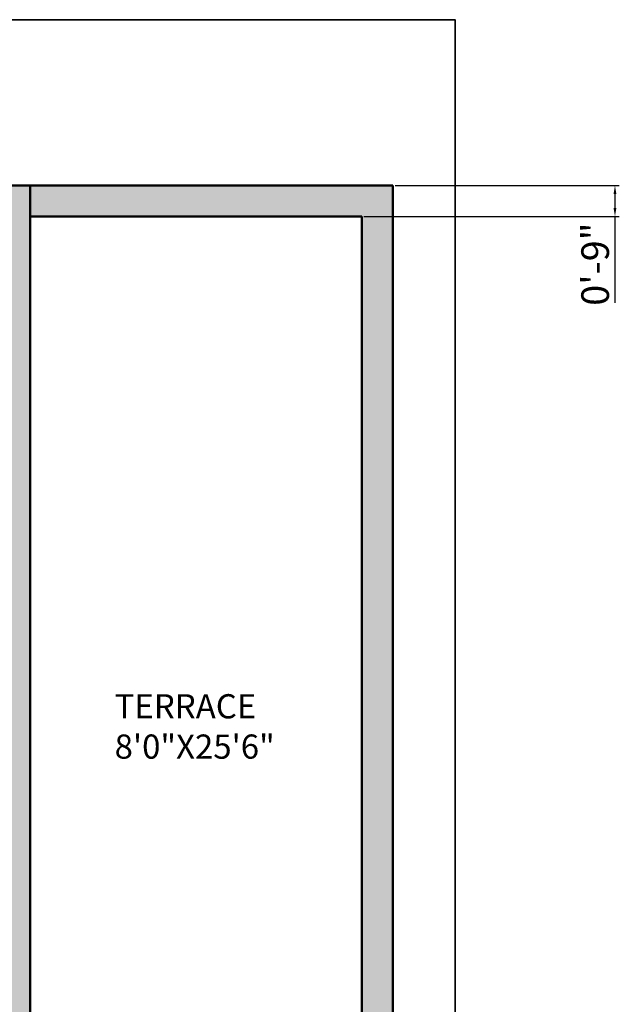
# Model space of a CAD drawing. Units: inches. Extents: x 1986 to 21484, y -1816 to 2016.
# Tile 45 of 85: x 2734 to 2908, y 1616 to 1901. Entities that reach past the tile are written whole.
import ezdxf

# ---------------------------------------------------------------- set-up
doc = ezdxf.new("R2010")
doc.units = ezdxf.units.IN
for name, color, linetype, lineweight in [('A-ANNO-DIMS', 2, 'Continuous', 18), ('A-AREA-IDEN', 3, 'Continuous', 18), ('A-WALL', 7, 'Continuous', 50), ('A-WALL-PATT', 8, 'Continuous', 13), ('C-PROP', 7, 'Continuous', 35)]:
    doc.layers.add(name, color=color, linetype=linetype, lineweight=lineweight)
doc.styles.get("Standard").update_dxf_attribs({"font": 'arial.ttf'})
doc.dimstyles.new('ISO-25', dxfattribs={"dimtxt": 8, "dimasz": 2.5, "dimexe": 1.25, "dimexo": 0.625, "dimtad": 1, "dimdec": 1, "dimlunit": 3, "dimtxsty": 'Standard', "dimcen": 2.5, "dimadec": 0, "dimazin": 0, "dimtfac": 1, "dimtdec": 1, "dimtmove": 0, "dimatfit": 3, "dimfxl": 1, "dimarcsym": 0})

# ---------------------------------------------------------------- blocks, each defined once
blk = doc.blocks.new('*D136')
at = {"layer": 'A-ANNO-DIMS', "color": 0, "lineweight": -2, "transparency": 16777216}
for p, q in [((2842.93, 1852.75), (2907.81, 1852.75)), ((2906.56, 1850.25), (2906.56, 1846.25)), ((2833.93, 1843.75), (2907.81, 1843.75)), ((2906.56, 1843.75), (2906.56, 1818.74))]:
    blk.add_line(p, q, dxfattribs=at)
at = {"layer": 'A-ANNO-DIMS', "color": 0, "transparency": 16777216}
for points in [[(2906.14, 1850.25), (2906.97, 1850.25), (2906.56, 1852.75)], [(2906.14, 1846.25), (2906.97, 1846.25), (2906.56, 1843.75)]]:
    blk.add_solid(points, dxfattribs=at)
at = {"layer": 'Defpoints', "color": 0, "transparency": 16777216}
for p in [(2842.31, 1852.75), (2833.31, 1843.75), (2906.56, 1843.75)]:
    blk.add_point(p, dxfattribs=at)
at = {"layer": 'A-ANNO-DIMS', "color": 0, "transparency": 16777216, "insert": (2901.85, 1829.99), "char_height": 8, "attachment_point": 5, "rotation": 90}
blk.add_mtext('0\'-9"', dxfattribs=at)

msp = doc.modelspace()

# ---------------------------------------------------------------- hatches: boundary and pattern name
at = {"layer": 'A-WALL-PATT'}
h = msp.add_hatch(color=256, dxfattribs=at)
h.dxf.hatch_style = 1
h.paths.add_polyline_path([(2545.31, 1843.75), (2665.31, 1843.75), (2665.31, 1852.75), (2536.31, 1852.75), (2536.31, 1765.75), (2545.31, 1765.75)])
h.paths.add_polyline_path([(2545.31, 1723.75), (2536.31, 1723.75), (2536.31, 1675.75), (2545.31, 1675.75), (2545.31, 1693.75), (2629.31, 1693.75), (2629.31, 1681.75), (2635.31, 1681.75), (2635.31, 1693.75), (2641.31, 1693.75), (2641.31, 1699.75), (2545.31, 1699.75)])
h.paths.add_polyline_path([(2545.31, 1651.75), (2536.31, 1651.75), (2536.31, 1615.75), (2545.31, 1615.75), (2545.31, 1627.75), (2695.31, 1627.75), (2695.31, 1699.75), (2671.31, 1699.75), (2671.31, 1693.75), (2689.31, 1693.75), (2689.31, 1633.75), (2635.31, 1633.75), (2635.31, 1651.75), (2629.31, 1651.75), (2629.31, 1633.75), (2545.31, 1633.75)])
h.paths.add_polyline_path([(2545.31, 1573.75), (2536.31, 1573.75), (2536.31, 1528.77), (2545.31, 1528.77)])
h.paths.add_polyline_path([(2545.31, 1486.77), (2536.31, 1486.77), (2536.31, 1441.75), (2545.31, 1441.75)])
h.paths.add_polyline_path([(2545.31, 1399.75), (2536.31, 1399.75), (2536.31, 1258.75), (2545.31, 1258.75)])
h.paths.add_polyline_path([(2609.81, 1387.75), (2581.31, 1387.75), (2581.31, 1378.75), (2609.81, 1378.75)])
h.paths.add_polyline_path([(2677.31, 1387.75), (2651.81, 1387.75), (2651.81, 1378.75), (2668.31, 1378.75), (2668.31, 1354.75), (2677.31, 1354.75)])
h.paths.add_polyline_path([(2842.31, 1387.75), (2833.31, 1387.75), (2713.31, 1387.75), (2713.31, 1381.75), (2833.31, 1381.75), (2833.31, 1363.75), (2842.31, 1363.75)])
h.paths.add_polyline_path([(2842.31, 1339.75), (2833.31, 1339.75), (2833.31, 1321.75), (2737.31, 1321.75), (2737.31, 1351.75), (2731.31, 1351.75), (2731.31, 1315.75), (2833.31, 1315.75), (2833.31, 1303.75), (2842.31, 1303.75)])
h.paths.add_polyline_path([(2677.31, 1312.75), (2668.31, 1312.75), (2668.31, 1189.75), (2677.31, 1189.75)])
h.paths.add_polyline_path([(2677.31, 1147.75), (2668.31, 1147.75), (2668.31, 1114.75), (2683.31, 1114.75), (2683.31, 1123.75), (2677.31, 1123.75)])
h.paths.add_polyline_path([(2842.31, 1147.75), (2833.31, 1147.75), (2833.31, 1123.75), (2725.31, 1123.75), (2725.31, 1114.75), (2842.31, 1114.75)])
h.paths.add_polyline_path([(2842.31, 1261.75), (2833.31, 1261.75), (2833.31, 1189.75), (2842.31, 1189.75)])
h.paths.add_polyline_path([(2842.31, 1441.75), (2833.31, 1441.75), (2833.31, 1423.75), (2842.31, 1423.75)])
h.paths.add_polyline_path([(2842.31, 1495.75), (2833.31, 1495.75), (2833.31, 1477.75), (2842.31, 1477.75)])
h.paths.add_polyline_path([(2737.31, 1852.75), (2707.31, 1852.75), (2707.31, 1843.75), (2731.31, 1843.75), (2731.31, 1573.75), (2737.31, 1573.75)])
h.paths.add_polyline_path([(2719.29, 1802.81), (2719.29, 1755.53), (2727.83, 1755.53), (2727.83, 1802.81)], flags=25)
h.paths.add_polyline_path([(2682.04, 1129.8), (2724.23, 1129.8), (2724.23, 1138.34), (2682.04, 1138.34)], flags=9)
h.paths.add_polyline_path([(2763.84, 1129.8), (2811.12, 1129.8), (2811.12, 1138.34), (2763.84, 1138.34)], flags=25)
h.paths.add_polyline_path([(2759.39, 1682.81), (2810.29, 1682.81), (2810.29, 1709.43), (2759.39, 1709.43)], flags=9)
h.paths.add_polyline_path([(2636.77, 1656.28), (2690.81, 1656.28), (2690.81, 1682.89), (2636.77, 1682.89)], flags=25)
h.paths.add_polyline_path([(2525.6, 1419.09), (2525.6, 1479.38), (2510.65, 1479.38), (2510.65, 1419.09)], flags=9)
h.paths.add_polyline_path([(2860.43, 1418.3), (2860.43, 1487.98), (2845.48, 1487.98), (2845.48, 1418.3)], flags=9)
h.paths.add_polyline_path([(2725.63, 1084.99), (2785.92, 1084.99), (2785.92, 1099.93), (2725.63, 1099.93)], flags=9)
h.paths.add_polyline_path([(2602.46, 1501.1), (2675.15, 1501.1), (2675.15, 1527.71), (2602.46, 1527.71)], flags=9)
h.paths.add_polyline_path([(2571.3, 1320.51), (2625.79, 1320.51), (2625.79, 1347.12), (2571.3, 1347.12)], flags=9)
h.paths.add_polyline_path([(2729.91, 1208.98), (2797.91, 1208.98), (2797.91, 1235.59), (2729.91, 1235.59)], flags=9)
h.paths.add_polyline_path([(2753.97, 1338.54), (2806.8, 1338.54), (2806.8, 1365.15), (2753.97, 1365.15)], flags=9)
h.paths.add_polyline_path([(2605.23, 1760.02), (2661.46, 1760.02), (2661.46, 1786.64), (2605.23, 1786.64)], flags=9)
h.paths.add_polyline_path([(2558.03, 1656.28), (2610.63, 1656.28), (2610.63, 1682.89), (2558.03, 1682.89)], flags=25)
h = msp.add_hatch(color=256, dxfattribs=at)
h.dxf.hatch_style = 1
h.paths.add_polyline_path([(2842.31, 1852.75), (2737.31, 1852.75), (2737.31, 1843.75), (2833.31, 1843.75), (2833.31, 1537.75), (2842.31, 1537.75)])
h.paths.add_polyline_path([(2682.04, 1129.8), (2724.23, 1129.8), (2724.23, 1138.34), (2682.04, 1138.34)], flags=9)
h.paths.add_polyline_path([(2763.84, 1129.8), (2811.12, 1129.8), (2811.12, 1138.34), (2763.84, 1138.34)], flags=9)
h.paths.add_polyline_path([(2719.29, 1802.81), (2719.29, 1755.53), (2727.83, 1755.53), (2727.83, 1802.81)], flags=9)
h.paths.add_polyline_path([(2759.39, 1682.81), (2810.29, 1682.81), (2810.29, 1709.43), (2759.39, 1709.43)], flags=25)
h.paths.add_polyline_path([(2636.77, 1656.28), (2690.81, 1656.28), (2690.81, 1682.89), (2636.77, 1682.89)], flags=9)
h.paths.add_polyline_path([(2525.6, 1419.09), (2525.6, 1479.38), (2510.65, 1479.38), (2510.65, 1419.09)], flags=9)
h.paths.add_polyline_path([(2860.43, 1418.3), (2860.43, 1487.98), (2845.48, 1487.98), (2845.48, 1418.3)], flags=9)
h.paths.add_polyline_path([(2725.63, 1084.99), (2785.92, 1084.99), (2785.92, 1099.93), (2725.63, 1099.93)], flags=9)
h.paths.add_polyline_path([(2602.46, 1501.1), (2675.15, 1501.1), (2675.15, 1527.71), (2602.46, 1527.71)], flags=9)
h.paths.add_polyline_path([(2571.3, 1320.51), (2625.79, 1320.51), (2625.79, 1347.12), (2571.3, 1347.12)], flags=9)
h.paths.add_polyline_path([(2710.58, 1210.46), (2778.57, 1210.46), (2778.57, 1237.07), (2710.58, 1237.07)], flags=9)
h.paths.add_polyline_path([(2753.97, 1338.54), (2806.8, 1338.54), (2806.8, 1365.15), (2753.97, 1365.15)], flags=9)
h.paths.add_polyline_path([(2605.23, 1728.88), (2661.46, 1728.88), (2661.46, 1755.49), (2605.23, 1755.49)], flags=9)
h.paths.add_polyline_path([(2558.03, 1656.28), (2610.63, 1656.28), (2610.63, 1682.89), (2558.03, 1682.89)], flags=9)

# ---------------------------------------------------------------- linework, layer by layer
at = {"layer": 'A-WALL'}
for p, q in [((2536.31, 1852.75), (2842.31, 1852.75)), ((2737.31, 1852.75), (2737.31, 1573.75)), ((2842.31, 1852.75), (2842.31, 1114.75)), ((2737.31, 1843.75), (2833.31, 1843.75)), ((2833.31, 1843.75), (2833.31, 1537.75))]:
    msp.add_line(p, q, dxfattribs=at)
at = {"layer": 'C-PROP'}
msp.add_lwpolyline([(2500.31, 1900.75), (2860.31, 1900.75), (2860.31, 1066.75), (2500.31, 1066.75)], close=True, dxfattribs=at)

# ---------------------------------------------------------------- texts
at = {"layer": 'A-AREA-IDEN', "insert": (2761.77, 1705.47), "char_height": 7, "attachment_point": 1}
msp.add_mtext_dynamic_manual_height_columns('{\\fTimes New Roman|b0|i0|c0|p18;TERRACE\\P8\'0"X25\'6"}', width=105.6127, gutter_width=12.5, heights=[0], dxfattribs=at)

# ---------------------------------------------------------------- dimensions: what is measured, and where the dimension line sits
at = {"layer": 'A-ANNO-DIMS'}
dim = msp.add_linear_dim(base=(2906.56, 1843.75), p1=(2842.31, 1852.75), p2=(2833.31, 1843.75), angle=90, dimstyle='ISO-25', override={"dimdec": 1, "dimlfac": 1, "dimrnd": 0, "dimzin": 1, "dimdsep": 46, "dimlunit": 4, "dimfrac": 2}, dxfattribs=at)
dim.commit()
dim.dimension.update_dxf_attribs({"geometry": '*D136', "text_midpoint": (2901.85, 1829.99)})

doc.saveas('drawing.dxf')
